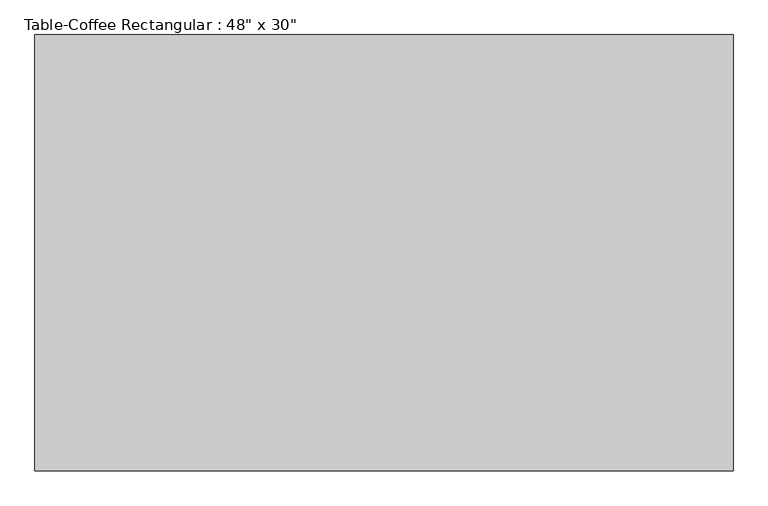
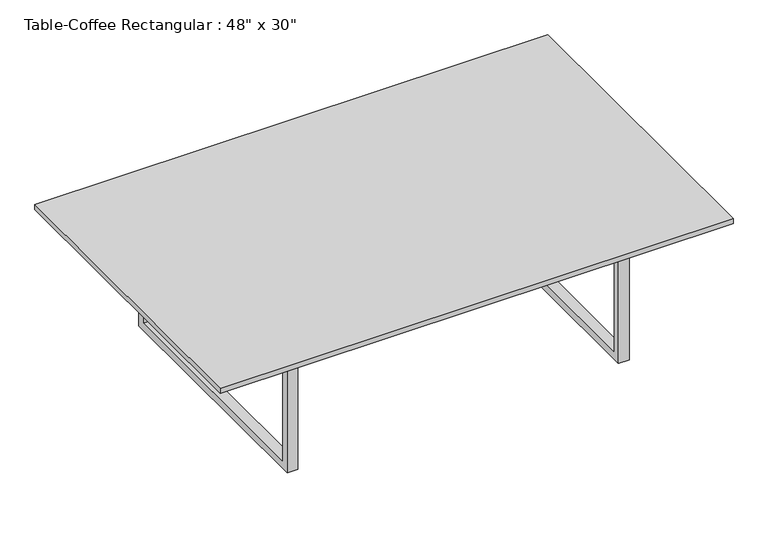
"""IFC4 building model written with IfcOpenShell, lengths in millimetres: furniture geometry."""

from ifc_helpers import new_model, si_unit, frame, origin, place, context, project, spatial, polyline, outline, extrude, source, transform, mapped, element, save


def furniture_acc2807d(model_context):
    return source(origin(), model_context, "Body", "SweptSolid", [
        extrude(outline(polyline([(1222.9336303, 750.6108318), (1222.9336303, -11.3891682), (3.7336303, -11.3891682), (3.7336303, 750.6108318), (1222.9336303, 750.6108318)])), frame((0.0, 0.0, 317.5), z_axis=(0.0, 0.0, 1.0), x_axis=(1.0, 0.0, 0.0)), (0.0, 0.0, 1.0), 12.7),
        extrude(outline(polyline([(64.8108318, 317.5), (674.4108318, 317.5), (674.4108318, 0.0), (64.8108318, 0.0), (64.8108318, 317.5)]), holes=[polyline([(83.8608318, 298.45), (83.8608318, 19.05), (655.3608318, 19.05), (655.3608318, 298.45), (83.8608318, 298.45)])]), frame((206.9336303, 0.0, 0.0), z_axis=(1.0, 0.0, 0.0), x_axis=(0.0, 1.0, 0.0)), (0.0, 0.0, 1.0), 25.4),
        extrude(outline(polyline([(64.8108318, 317.5), (674.4108318, 317.5), (674.4108318, 0.0), (64.8108318, 0.0), (64.8108318, 317.5)]), holes=[polyline([(83.8608318, 298.45), (83.8608318, 19.05), (655.3608318, 19.05), (655.3608318, 298.45), (83.8608318, 298.45)])]), frame((994.3336303, 0.0, 0.0), z_axis=(1.0, 0.0, 0.0), x_axis=(0.0, 1.0, 0.0)), (0.0, 0.0, 1.0), 25.4),
        extrude(outline(polyline([(994.3336303, 379.1358318), (994.3336303, 360.0858318), (232.3336303, 360.0858318), (232.3336303, 379.1358318), (994.3336303, 379.1358318)])), frame((0.0, 0.0, 298.45), z_axis=(0.0, 0.0, 1.0), x_axis=(1.0, 0.0, 0.0)), (0.0, 0.0, 1.0), 19.05),
    ])


if __name__ == "__main__":
    model = new_model("IFC4")
    model_context = context("Model", 3, world=origin())
    ifc_project = project(units=[si_unit("LENGTHUNIT", "METRE", prefix="MILLI")], contexts=[model_context])
    site = spatial("IfcSite", under=ifc_project)
    building = spatial("IfcBuilding", under=site)
    placement = place(None, origin())
    furniture_shape = furniture_acc2807d(model_context)
    element("IfcFurniture", 1, ObjectType="Table-Coffee Rectangular : 48\" x 30\"", at=placement, inside=building, context=model_context, shape_type="MappedRepresentation", body=[
        mapped(furniture_shape, transform((0.0, 0.0, 0.0), x_axis=(1.0, 0.0, 0.0), y_axis=(0.0, 1.0, 0.0), z_axis=(0.0, 0.0, 1.0))),
    ])
    save(model, "model.ifc")

# Revit data of these elements
# Type "Table-Coffee Rectangular : 48\" x 30\""
#   Assembly Code = "E2020200"
#   Height = 1' - 1"
#   Length = 4' - 0"
#   Width = 2' - 6"
#   Base Material = Metal - Chrome
#   Table Top Material = Glass - Clear, Grey
#   Default Elevation = 0
# Element 1 (IfcFurniture, "Table-Coffee Rectangular : 48\" x 30\"")
#   Materials on its faces: "Metal - Chrome", "Glass - Clear, Grey"
# Materials
#   "Metal - Chrome": colour RGB 57 57 57, transparency 0
#   "Glass - Clear, Grey": colour RGB 252 255 255, transparency 0.64
